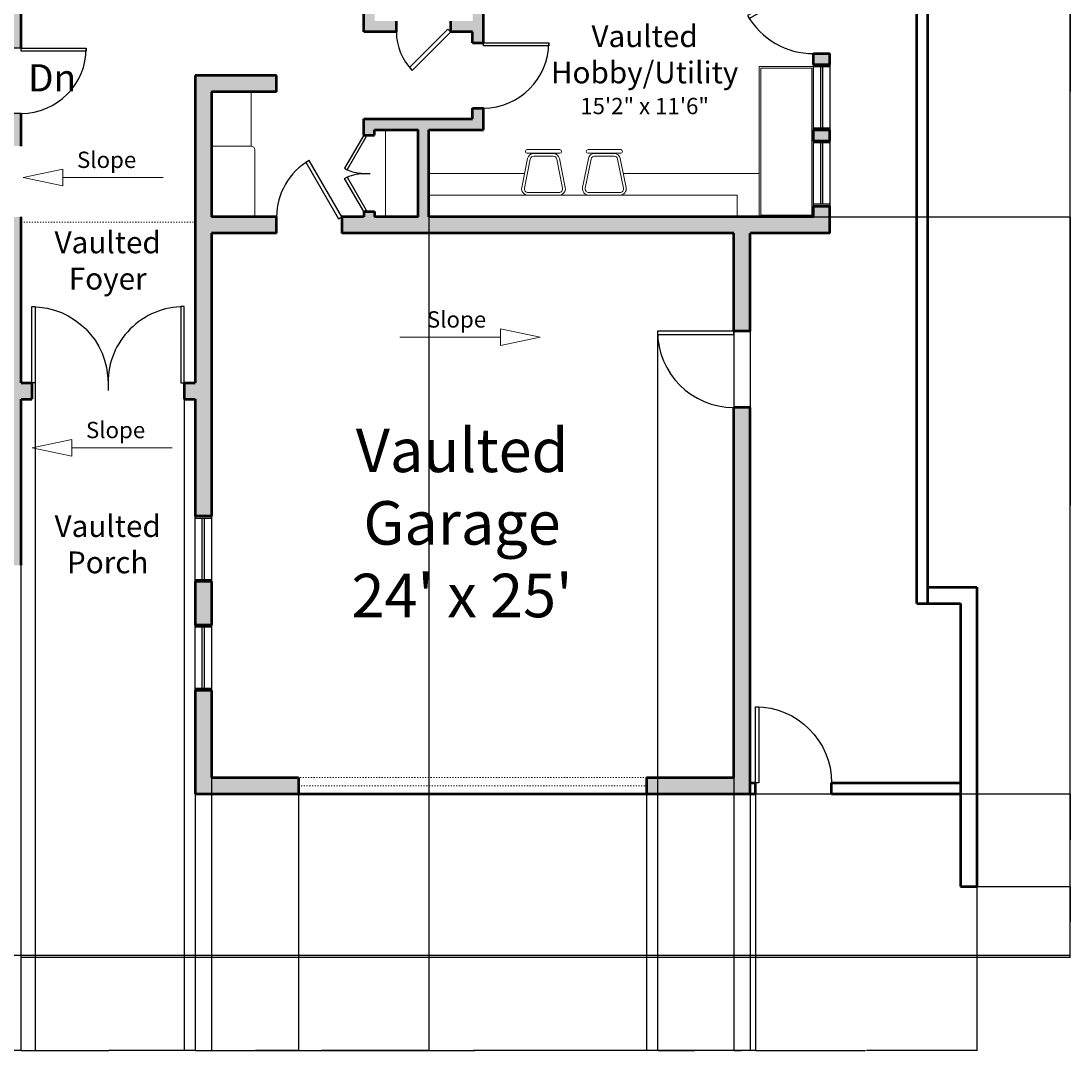
# Model space of a CAD drawing. Units: inches. Extents: x 296 to 2116, y 330 to 1460.
# Tile 2 of 9: x 657 to 1235, y 330 to 898. Entities that reach past the tile are written whole.
import ezdxf

# ---------------------------------------------------------------- set-up
doc = ezdxf.new("R2010")
doc.units = ezdxf.units.IN
doc.linetypes.add('ACAD_ISO03W100', pattern=[30, 12, -18])
for name, color, linetype, lineweight in [('A-ANNO-DIMS', 2, 'Continuous', 18), ('A-ANNO-SYMB', 2, 'Continuous', 18), ('A-ANNO-TEXT', 7, 'Continuous', 18), ('A-AREA-IDEN', 7, 'Continuous', 25), ('A-DOOR', 3, 'Continuous', 25), ('A-FLOR-FIXT', 8, 'Continuous', 18), ('A-FLOR-OVHD', 132, 'ACAD_ISO03W100', 18), ('A-GLAZ', 4, 'Continuous', 25), ('A-WALL', 7, 'Continuous', 50), ('A-WALL-PATT', 8, 'Continuous', 13)]:
    doc.layers.add(name, color=color, linetype=linetype, lineweight=lineweight)
doc.styles.get("Standard").update_dxf_attribs({"font": 'arial.ttf'})
doc.dimstyles.get("Standard").update_dxf_attribs({"dimtxt": 0.18, "dimasz": 0.18, "dimexe": 0.18, "dimexo": 0.0625, "dimgap": 0.09, "dimtad": 0, "dimtih": 1, "dimtoh": 1, "dimdec": 4, "dimzin": 0, "dimdsep": 46, "dimtxsty": 'Standard', "dimcen": 0.09, "dimadec": 0, "dimazin": 0, "dimtfac": 1, "dimtdec": 4, "dimtofl": 0, "dimtmove": 0, "dimatfit": 3, "dimfxl": 1, "dimtolj": 1, "dimtzin": 0, "dimarcsym": 0})

# ---------------------------------------------------------------- blocks, each defined once
blk = doc.blocks.new('*U5')
for p, q in [((0, 0), (0, 4)), ((40, 0), (40, 4))]:
    blk.add_line(p, q)
blk.add_lwpolyline([(0, 0), (0, -40), (1.75, -40), (1.75, 0)], close=True)
blk.add_arc((0, 0), 40, 270, 0)
blk = doc.blocks.new('*U6')
for p, q in [((0, 0), (0, 4)), ((30, 0), (30, 4))]:
    blk.add_line(p, q)
blk.add_lwpolyline([(0, 0), (15, -25.98), (16.52, -25.11), (1.52, 0.88)], close=True)
blk.add_arc((0, 0), 30, 300, 0)
blk = doc.blocks.new('*U8')
for p, q in [((-24, 0), (-24, -4)), ((0, 0), (0, -4))]:
    blk.add_line(p, q)
blk.add_lwpolyline([(0, 0), (-20.78, 12), (-21.66, 10.48), (-0.88, -1.52)], close=True)
blk.add_arc((0, 0), 24, 150, 180)
blk = doc.blocks.new('*U7')
for p, q in [((-36, 0), (-36, 4)), ((0, 0), (0, 4))]:
    blk.add_line(p, q)
blk.add_lwpolyline([(0, 0), (0, -36), (-1.75, -36), (-1.75, 0)], close=True)
blk.add_arc((0, 0), 36, 180, 270)
blk = doc.blocks.new('*U10')
for p, q in [((0, 0), (0, -4)), ((24, 0), (24, -4))]:
    blk.add_line(p, q)
blk.add_lwpolyline([(0, 0), (16.97, 16.97), (18.21, 15.73), (1.24, -1.24)], close=True)
blk.add_arc((0, 0), 24, 0, 45)
blk = doc.blocks.new('*U11')
for p, q in [((0, 0), (0, -4)), ((-40, 0), (-40, -4))]:
    blk.add_line(p, q)
blk.add_lwpolyline([(0, 0), (-20, 34.64), (-21.52, 33.77), (-1.52, -0.88)], close=True)
blk.add_arc((0, 0), 40, 120, 180)
blk = doc.blocks.new('*U12')
for p, q in [((0, 0), (0, -4)), ((-40, 0), (-40, -4))]:
    blk.add_line(p, q)
blk.add_lwpolyline([(0, 0), (0, 40), (-1.75, 40), (-1.75, 0)], close=True)
blk.add_arc((0, 0), 40, 90, 180)
blk = doc.blocks.new('*U15')
for p, q in [((-36, 0), (-36, 6)), ((0, 0), (0, 6))]:
    blk.add_line(p, q)
blk.add_lwpolyline([(0, 0), (0, -36), (-1.75, -36), (-1.75, 0)], close=True)
blk.add_arc((0, 0), 36, 180, 270)
blk = doc.blocks.new('SLOPE-ARROW')
blk.add_line((739.99, 662.71), (684.54, 662.71))
blk.add_lwpolyline([(662.67, 662.71), (684.54, 658.1), (684.54, 667.32)], close=True)
blk = doc.blocks.new('*D45')
at = {"layer": 'A-ANNO-DIMS', "color": 0, "lineweight": -2, "transparency": 16777216}
for p, q in [((1156.58, 1407.95), (1235.3, 1407.95)), ((1235.12, 1407.77), (1235.12, 895.66)), ((1235.12, 383.18), (1235.12, 895.29)), ((609.63, 383), (1235.3, 383))]:
    blk.add_line(p, q, dxfattribs=at)
at = {"layer": 'A-ANNO-DIMS', "color": 0, "transparency": 16777216}
for points in [[(1235.09, 1407.77), (1235.15, 1407.77), (1235.12, 1407.95)], [(1235.09, 383.18), (1235.15, 383.18), (1235.12, 383)]]:
    blk.add_solid(points, dxfattribs=at)
at = {"layer": 'Defpoints', "color": 0, "transparency": 16777216}
for p in [(1156.52, 1407.95), (1235.12, 1407.95), (609.57, 383)]:
    blk.add_point(p, dxfattribs=at)
at = {"layer": 'A-ANNO-DIMS', "color": 0, "transparency": 16777216, "insert": (1235.12, 895.48), "char_height": 0.18, "attachment_point": 5}
blk.add_mtext('\\A1;1025', dxfattribs=at)
blk = doc.blocks.new('*D53')
at = {"layer": 'A-ANNO-DIMS', "color": 0, "lineweight": -2, "transparency": 16777216}
for p, q in [((609.57, 382.94), (609.57, 330.22)), ((656.57, 381.94), (656.57, 330.22)), ((609.75, 330.4), (632.85, 330.4)), ((656.39, 330.4), (633.29, 330.4))]:
    blk.add_line(p, q, dxfattribs=at)
at = {"layer": 'A-ANNO-DIMS', "color": 0, "transparency": 16777216}
for points in [[(609.75, 330.43), (609.75, 330.37), (609.57, 330.4)], [(656.39, 330.43), (656.39, 330.37), (656.57, 330.4)]]:
    blk.add_solid(points, dxfattribs=at)
at = {"layer": 'Defpoints', "color": 0, "transparency": 16777216}
for p in [(609.57, 383), (656.57, 382), (656.57, 330.4)]:
    blk.add_point(p, dxfattribs=at)
at = {"layer": 'A-ANNO-DIMS', "color": 0, "transparency": 16777216, "insert": (633.07, 330.4), "char_height": 0.18, "attachment_point": 5}
blk.add_mtext('\\A1;47', dxfattribs=at)
blk = doc.blocks.new('*D54')
at = {"layer": 'A-ANNO-DIMS', "color": 0, "lineweight": -2, "transparency": 16777216}
for p, q in [((656.57, 597.94), (656.57, 330.22)), ((752.52, 471.89), (752.52, 330.22)), ((656.75, 330.4), (704.15, 330.4)), ((752.34, 330.4), (704.94, 330.4))]:
    blk.add_line(p, q, dxfattribs=at)
at = {"layer": 'A-ANNO-DIMS', "color": 0, "transparency": 16777216}
for points in [[(656.75, 330.43), (656.75, 330.37), (656.57, 330.4)], [(752.34, 330.43), (752.34, 330.37), (752.52, 330.4)]]:
    blk.add_solid(points, dxfattribs=at)
at = {"layer": 'Defpoints', "color": 0, "transparency": 16777216}
for p in [(656.57, 598), (752.52, 471.95), (752.52, 330.4)]:
    blk.add_point(p, dxfattribs=at)
at = {"layer": 'A-ANNO-DIMS', "color": 0, "transparency": 16777216, "insert": (704.55, 330.4), "char_height": 0.18, "attachment_point": 5}
blk.add_mtext('\\A1;95.95', dxfattribs=at)
blk = doc.blocks.new('*D55')
at = {"layer": 'A-ANNO-DIMS', "color": 0, "lineweight": -2, "transparency": 16777216}
for p, q in [((752.52, 471.89), (752.52, 330.22)), ((1061.52, 471.89), (1061.52, 330.22)), ((752.7, 330.4), (906.73, 330.4)), ((1061.34, 330.4), (907.31, 330.4))]:
    blk.add_line(p, q, dxfattribs=at)
at = {"layer": 'A-ANNO-DIMS', "color": 0, "transparency": 16777216}
for points in [[(752.7, 330.43), (752.7, 330.37), (752.52, 330.4)], [(1061.34, 330.43), (1061.34, 330.37), (1061.52, 330.4)]]:
    blk.add_solid(points, dxfattribs=at)
at = {"layer": 'Defpoints', "color": 0, "transparency": 16777216}
for p in [(752.52, 471.95), (1061.52, 471.95), (1061.52, 330.4)]:
    blk.add_point(p, dxfattribs=at)
at = {"layer": 'A-ANNO-DIMS', "color": 0, "transparency": 16777216, "insert": (907.02, 330.4), "char_height": 0.18, "attachment_point": 5}
blk.add_mtext('\\A1;309', dxfattribs=at)
blk = doc.blocks.new('*D56')
at = {"layer": 'A-ANNO-DIMS', "color": 0, "lineweight": -2, "transparency": 16777216}
for p, q in [((1183.52, 585.89), (1183.52, 330.22)), ((1061.52, 471.89), (1061.52, 330.22)), ((1061.7, 330.4), (1122.24, 330.4)), ((1183.34, 330.4), (1122.8, 330.4))]:
    blk.add_line(p, q, dxfattribs=at)
at = {"layer": 'A-ANNO-DIMS', "color": 0, "transparency": 16777216}
for points in [[(1061.7, 330.43), (1061.7, 330.37), (1061.52, 330.4)], [(1183.34, 330.43), (1183.34, 330.37), (1183.52, 330.4)]]:
    blk.add_solid(points, dxfattribs=at)
at = {"layer": 'Defpoints', "color": 0, "transparency": 16777216}
for p in [(1183.52, 585.95), (1061.52, 471.95), (1183.52, 330.4)]:
    blk.add_point(p, dxfattribs=at)
at = {"layer": 'A-ANNO-DIMS', "color": 0, "transparency": 16777216, "insert": (1122.52, 330.4), "char_height": 0.18, "attachment_point": 5}
blk.add_mtext('\\A1;122', dxfattribs=at)
blk = doc.blocks.new('*D60')
at = {"layer": 'A-ANNO-DIMS', "color": 0, "lineweight": -2, "transparency": 16777216}
for p, q in [((1174.58, 420.95), (1235.3, 420.95)), ((1235.12, 420.77), (1235.12, 401.66)), ((1235.12, 382.18), (1235.12, 401.29)), ((656.63, 382), (1235.3, 382))]:
    blk.add_line(p, q, dxfattribs=at)
at = {"layer": 'A-ANNO-DIMS', "color": 0, "transparency": 16777216}
for points in [[(1235.09, 420.77), (1235.15, 420.77), (1235.12, 420.95)], [(1235.09, 382.18), (1235.15, 382.18), (1235.12, 382)]]:
    blk.add_solid(points, dxfattribs=at)
at = {"layer": 'Defpoints', "color": 0, "transparency": 16777216}
for p in [(1174.52, 420.95), (1235.12, 420.95), (656.57, 382)]:
    blk.add_point(p, dxfattribs=at)
at = {"layer": 'A-ANNO-DIMS', "color": 0, "transparency": 16777216, "insert": (1235.12, 401.48), "char_height": 0.18, "attachment_point": 5}
blk.add_mtext('\\A1;38.955', dxfattribs=at)
blk = doc.blocks.new('*D61')
at = {"layer": 'A-ANNO-DIMS', "color": 0, "lineweight": -2, "transparency": 16777216}
for p, q in [((1061.58, 471.95), (1235.3, 471.95)), ((1235.12, 471.77), (1235.12, 446.64)), ((1235.12, 421.13), (1235.12, 446.27)), ((1174.58, 420.95), (1235.3, 420.95))]:
    blk.add_line(p, q, dxfattribs=at)
at = {"layer": 'A-ANNO-DIMS', "color": 0, "transparency": 16777216}
for points in [[(1235.09, 471.77), (1235.15, 471.77), (1235.12, 471.95)], [(1235.09, 421.13), (1235.15, 421.13), (1235.12, 420.95)]]:
    blk.add_solid(points, dxfattribs=at)
at = {"layer": 'Defpoints', "color": 0, "transparency": 16777216}
for p in [(1061.52, 471.95), (1235.12, 471.95), (1174.52, 420.95)]:
    blk.add_point(p, dxfattribs=at)
at = {"layer": 'A-ANNO-DIMS', "color": 0, "transparency": 16777216, "insert": (1235.12, 446.45), "char_height": 0.18, "attachment_point": 5}
blk.add_mtext('\\A1;51', dxfattribs=at)
blk = doc.blocks.new('*D62')
at = {"layer": 'A-ANNO-DIMS', "color": 0, "lineweight": -2, "transparency": 16777216}
for p, q in [((1063.58, 789.95), (1235.3, 789.95)), ((1235.12, 789.77), (1235.12, 631.14)), ((1235.12, 472.13), (1235.12, 630.77)), ((1061.58, 471.95), (1235.3, 471.95))]:
    blk.add_line(p, q, dxfattribs=at)
at = {"layer": 'A-ANNO-DIMS', "color": 0, "transparency": 16777216}
for points in [[(1235.09, 789.77), (1235.15, 789.77), (1235.12, 789.95)], [(1235.09, 472.13), (1235.15, 472.13), (1235.12, 471.95)]]:
    blk.add_solid(points, dxfattribs=at)
at = {"layer": 'Defpoints', "color": 0, "transparency": 16777216}
for p in [(1063.52, 789.95), (1235.12, 789.95), (1061.52, 471.95)]:
    blk.add_point(p, dxfattribs=at)
at = {"layer": 'A-ANNO-DIMS', "color": 0, "transparency": 16777216, "insert": (1235.12, 630.95), "char_height": 0.18, "attachment_point": 5}
blk.add_mtext('\\A1;318', dxfattribs=at)
blk = doc.blocks.new('*D63')
at = {"layer": 'A-ANNO-DIMS', "color": 0, "lineweight": -2, "transparency": 16777216}
for p, q in [((1102.58, 1156.95), (1235.3, 1156.95)), ((1235.12, 1156.77), (1235.12, 973.64)), ((1235.12, 790.13), (1235.12, 973.27)), ((1063.58, 789.95), (1235.3, 789.95))]:
    blk.add_line(p, q, dxfattribs=at)
at = {"layer": 'A-ANNO-DIMS', "color": 0, "transparency": 16777216}
for points in [[(1235.09, 1156.77), (1235.15, 1156.77), (1235.12, 1156.95)], [(1235.09, 790.13), (1235.15, 790.13), (1235.12, 789.95)]]:
    blk.add_solid(points, dxfattribs=at)
at = {"layer": 'Defpoints', "color": 0, "transparency": 16777216}
for p in [(1102.52, 1156.95), (1235.12, 1156.95), (1063.52, 789.95)]:
    blk.add_point(p, dxfattribs=at)
at = {"layer": 'A-ANNO-DIMS', "color": 0, "transparency": 16777216, "insert": (1235.12, 973.45), "char_height": 0.18, "attachment_point": 5}
blk.add_mtext('\\A1;367', dxfattribs=at)
blk = doc.blocks.new('*D76')
at = {"layer": 'A-ANNO-DIMS', "color": 0, "lineweight": -2, "transparency": 16777216}
for p, q in [((1049.52, 780.89), (1049.52, 330.22)), ((1058.52, 780.89), (1058.52, 330.22)), ((1049.7, 330.4), (1053.7, 330.4)), ((1058.34, 330.4), (1054.35, 330.4))]:
    blk.add_line(p, q, dxfattribs=at)
at = {"layer": 'A-ANNO-DIMS', "color": 0, "transparency": 16777216}
for points in [[(1049.7, 330.43), (1049.7, 330.37), (1049.52, 330.4)], [(1058.34, 330.43), (1058.34, 330.37), (1058.52, 330.4)]]:
    blk.add_solid(points, dxfattribs=at)
at = {"layer": 'Defpoints', "color": 0, "transparency": 16777216}
for p in [(1049.52, 780.95), (1058.52, 780.95), (1058.52, 330.4)]:
    blk.add_point(p, dxfattribs=at)
at = {"layer": 'A-ANNO-DIMS', "color": 0, "transparency": 16777216, "insert": (1054.02, 330.4), "char_height": 0.18, "attachment_point": 5}
blk.add_mtext('\\A1;9.00', dxfattribs=at)
blk = doc.blocks.new('*D95')
at = {"layer": 'A-ANNO-DIMS', "color": 0, "lineweight": -2, "transparency": 16777216}
for p, q in [((761.52, 480.89), (761.52, 330.22)), ((809.52, 480.89), (809.52, 330.22)), ((761.7, 330.4), (785.13, 330.4)), ((809.34, 330.4), (785.92, 330.4))]:
    blk.add_line(p, q, dxfattribs=at)
at = {"layer": 'A-ANNO-DIMS', "color": 0, "transparency": 16777216}
for points in [[(761.7, 330.43), (761.7, 330.37), (761.52, 330.4)], [(809.34, 330.43), (809.34, 330.37), (809.52, 330.4)]]:
    blk.add_solid(points, dxfattribs=at)
at = {"layer": 'Defpoints', "color": 0, "transparency": 16777216}
for p in [(761.52, 480.95), (809.52, 480.95), (809.52, 330.4)]:
    blk.add_point(p, dxfattribs=at)
at = {"layer": 'A-ANNO-DIMS', "color": 0, "transparency": 16777216, "insert": (785.52, 330.4), "char_height": 0.18, "attachment_point": 5}
blk.add_mtext('\\A1;48.00', dxfattribs=at)
blk = doc.blocks.new('*D96')
at = {"layer": 'A-ANNO-DIMS', "color": 0, "lineweight": -2, "transparency": 16777216}
for p, q in [((809.52, 480.89), (809.52, 330.22)), ((1001.52, 480.89), (1001.52, 330.22)), ((809.7, 330.4), (905.07, 330.4)), ((1001.34, 330.4), (905.98, 330.4))]:
    blk.add_line(p, q, dxfattribs=at)
at = {"layer": 'A-ANNO-DIMS', "color": 0, "transparency": 16777216}
for points in [[(809.7, 330.43), (809.7, 330.37), (809.52, 330.4)], [(1001.34, 330.43), (1001.34, 330.37), (1001.52, 330.4)]]:
    blk.add_solid(points, dxfattribs=at)
at = {"layer": 'Defpoints', "color": 0, "transparency": 16777216}
for p in [(809.52, 480.95), (1001.52, 480.95), (1001.52, 330.4)]:
    blk.add_point(p, dxfattribs=at)
at = {"layer": 'A-ANNO-DIMS', "color": 0, "transparency": 16777216, "insert": (905.52, 330.4), "char_height": 0.18, "attachment_point": 5}
blk.add_mtext('\\A1;192.00', dxfattribs=at)
blk = doc.blocks.new('*D97')
at = {"layer": 'A-ANNO-DIMS', "color": 0, "lineweight": -2, "transparency": 16777216}
for p, q in [((881.52, 789.89), (881.52, 330.22)), ((761.52, 780.89), (761.52, 330.22)), ((761.7, 330.4), (821.07, 330.4)), ((881.34, 330.4), (821.98, 330.4))]:
    blk.add_line(p, q, dxfattribs=at)
at = {"layer": 'A-ANNO-DIMS', "color": 0, "transparency": 16777216}
for points in [[(761.7, 330.43), (761.7, 330.37), (761.52, 330.4)], [(881.34, 330.43), (881.34, 330.37), (881.52, 330.4)]]:
    blk.add_solid(points, dxfattribs=at)
at = {"layer": 'Defpoints', "color": 0, "transparency": 16777216}
for p in [(881.52, 789.95), (761.52, 780.95), (881.52, 330.4)]:
    blk.add_point(p, dxfattribs=at)
at = {"layer": 'A-ANNO-DIMS', "color": 0, "transparency": 16777216, "insert": (821.52, 330.4), "char_height": 0.18, "attachment_point": 5}
blk.add_mtext('\\A1;120.00', dxfattribs=at)
blk = doc.blocks.new('*D98')
at = {"layer": 'A-ANNO-DIMS', "color": 0, "lineweight": -2, "transparency": 16777216}
for p, q in [((1030.58, 927.95), (1235.3, 927.95)), ((1235.12, 927.77), (1235.12, 859.14)), ((1235.12, 790.13), (1235.12, 858.77)), ((1093.58, 789.95), (1235.3, 789.95))]:
    blk.add_line(p, q, dxfattribs=at)
at = {"layer": 'A-ANNO-DIMS', "color": 0, "transparency": 16777216}
for points in [[(1235.09, 927.77), (1235.15, 927.77), (1235.12, 927.95)], [(1235.09, 790.13), (1235.15, 790.13), (1235.12, 789.95)]]:
    blk.add_solid(points, dxfattribs=at)
at = {"layer": 'Defpoints', "color": 0, "transparency": 16777216}
for p in [(1030.52, 927.95), (1235.12, 927.95), (1093.52, 789.95)]:
    blk.add_point(p, dxfattribs=at)
at = {"layer": 'A-ANNO-DIMS', "color": 0, "transparency": 16777216, "insert": (1235.12, 858.95), "char_height": 0.18, "attachment_point": 5}
blk.add_mtext('\\A1;138.00', dxfattribs=at)
blk = doc.blocks.new('*D99')
at = {"layer": 'A-ANNO-DIMS', "color": 0, "lineweight": -2, "transparency": 16777216}
for p, q in [((664.38, 698.44), (664.38, 330.22)), ((746.55, 698.44), (746.55, 330.22)), ((664.56, 330.4), (705.07, 330.4)), ((746.37, 330.4), (705.86, 330.4))]:
    blk.add_line(p, q, dxfattribs=at)
at = {"layer": 'A-ANNO-DIMS', "color": 0, "transparency": 16777216}
for points in [[(664.56, 330.43), (664.56, 330.37), (664.38, 330.4)], [(746.37, 330.43), (746.37, 330.37), (746.55, 330.4)]]:
    blk.add_solid(points, dxfattribs=at)
at = {"layer": 'Defpoints', "color": 0, "transparency": 16777216}
for p in [(664.38, 698.5), (746.55, 698.5), (746.55, 330.4)]:
    blk.add_point(p, dxfattribs=at)
at = {"layer": 'A-ANNO-DIMS', "color": 0, "transparency": 16777216, "insert": (705.47, 330.4), "char_height": 0.18, "attachment_point": 5}
blk.add_mtext('\\A1;82.16', dxfattribs=at)
blk = doc.blocks.new('*D101')
at = {"layer": 'A-ANNO-DIMS', "color": 0, "lineweight": -2, "transparency": 16777216}
for p, q in [((1007.52, 726.89), (1007.52, 330.22)), ((1049.52, 726.89), (1049.52, 330.22)), ((1007.7, 330.4), (1028.13, 330.4)), ((1049.34, 330.4), (1028.92, 330.4))]:
    blk.add_line(p, q, dxfattribs=at)
at = {"layer": 'A-ANNO-DIMS', "color": 0, "transparency": 16777216}
for points in [[(1007.7, 330.43), (1007.7, 330.37), (1007.52, 330.4)], [(1049.34, 330.43), (1049.34, 330.37), (1049.52, 330.4)]]:
    blk.add_solid(points, dxfattribs=at)
at = {"layer": 'Defpoints', "color": 0, "transparency": 16777216}
for p in [(1007.52, 726.95), (1049.52, 726.95), (1049.52, 330.4)]:
    blk.add_point(p, dxfattribs=at)
at = {"layer": 'A-ANNO-DIMS', "color": 0, "transparency": 16777216, "insert": (1028.52, 330.4), "char_height": 0.18, "attachment_point": 5}
blk.add_mtext('\\A1;42.00', dxfattribs=at)

msp = doc.modelspace()

# ---------------------------------------------------------------- hatches: boundary and pattern name
at = {"layer": 'A-WALL-PATT'}
h = msp.add_hatch(color=256, dxfattribs=at)
h.dxf.hatch_style = 1
h.paths.add_polyline_path([(656.5723, 927.9991), (668.5723, 927.9991), (668.5723, 936.9991), (650.5723, 936.9991), (650.5723, 897.9991), (356.5223, 897.9991), (356.5223, 955.9991), (347.5223, 955.9991), (347.5223, 888.9991), (423.5723, 888.9991), (423.5723, 766.9991), (432.5723, 766.9991), (432.5723, 834.9991), (453.5723, 834.9991), (468.5723, 834.9991), (468.5723, 840.9991), (432.5723, 840.9991), (432.5723, 888.9991), (504.5723, 888.9991), (504.5723, 840.9991), (504.5723, 834.9991), (531.6223, 834.9991), (531.6223, 768.5344), (527.8443, 764.7564), (530.6728, 761.928), (532.087, 760.5138), (540.5723, 768.9991), (598.0723, 768.9991), (598.0723, 777.9991), (601.8223, 777.9991), (601.8223, 782.1991), (601.8223, 783.9991), (598.0723, 783.9991), (598.0723, 798.9991), (592.0723, 798.9991), (592.0723, 774.9991), (537.6223, 774.9991), (537.6223, 834.9991), (592.0723, 834.9991), (592.0723, 828.9991), (598.0723, 828.9991), (598.0723, 834.9991), (647.5723, 834.9991), (647.5723, 828.9991), (656.5723, 828.9991), (656.5723, 846.9991), (650.5723, 846.9991), (647.5723, 846.9991), (647.5723, 840.9991), (510.5723, 840.9991), (510.5723, 888.9991), (647.5723, 888.9991), (647.5723, 882.9991), (656.5723, 882.9991)])
h.paths.add_polyline_path([(432.5723, 730.9991), (496.5723, 730.9991), (496.5723, 724.9991), (502.5723, 724.9991), (502.5723, 730.9991), (506.6311, 735.058), (502.3885, 739.3006), (500.087, 736.9991), (432.5723, 736.9991), (432.5723, 742.9991), (423.5723, 742.9991), (423.5723, 641.9991), (490.5723, 641.9991), (490.5723, 597.9991), (531.5723, 597.9991), (531.5723, 606.9991), (499.5723, 606.9991), (499.5723, 650.9991), (502.5723, 650.9991), (502.5723, 659.9991), (496.5723, 659.9991), (493.5723, 659.9991), (493.5723, 650.9991), (432.5723, 650.9991)])
h.paths.add_polyline_path([(656.5723, 689.4991), (662.5473, 689.4991), (662.5473, 698.4991), (656.5723, 698.4991), (656.5723, 789.9991), (647.5723, 789.9991), (647.5723, 783.9991), (643.8223, 783.9991), (643.8223, 777.9991), (647.5723, 777.9991), (647.5723, 606.9991), (615.5723, 606.9991), (615.5723, 597.9991), (656.5723, 597.9991)])
h.paths.add_polyline_path([(761.5223, 780.9541), (797.5223, 780.9541), (797.5223, 789.9541), (761.5223, 789.9541), (761.5223, 858.9541), (797.5223, 858.9541), (797.5223, 867.9541), (752.5223, 867.9541), (752.5223, 698.4991), (746.5473, 698.4991), (746.5473, 694.2991), (746.5473, 689.4991), (752.5223, 689.4991), (752.5223, 624.9541), (761.5223, 624.9541)])
h.paths.add_polyline_path([(1102.5223, 795.9541), (1093.5223, 795.9541), (1093.5223, 789.9541), (1063.5223, 789.9541), (881.5223, 789.9541), (881.5223, 837.9541), (911.5223, 837.9541), (911.5223, 849.9541), (907.5223, 849.9541), (905.5223, 849.9541), (905.5223, 843.9541), (845.5223, 843.9541), (845.5223, 834.9541), (849.0223, 834.9541), (851.5223, 834.9541), (851.5223, 837.9541), (875.5223, 837.9541), (875.5223, 789.9541), (851.5223, 789.9541), (851.5223, 792.9541), (845.5223, 792.9541), (845.5223, 789.9541), (833.5223, 789.9541), (833.5223, 785.1541), (833.5223, 780.9541), (1049.5223, 780.9541), (1049.5223, 726.9541), (1053.7223, 726.9541), (1058.5223, 726.9541), (1058.5223, 780.9541), (1102.5223, 780.9541)])
h.paths.add_polyline_path([(761.5223, 588.9541), (752.5223, 588.9541), (752.5223, 564.9541), (761.5223, 564.9541)])
h.paths.add_polyline_path([(809.5223, 480.9541), (761.5223, 480.9541), (761.5223, 528.9541), (752.5223, 528.9541), (752.5223, 471.9541), (809.5223, 471.9541)])
h.paths.add_polyline_path([(1058.5223, 684.9541), (1049.5223, 684.9541), (1049.5223, 480.9541), (1001.5223, 480.9541), (1001.5223, 476.4541), (1001.5223, 471.9541), (1058.5223, 471.9541)])
h.paths.add_polyline_path([(794.5223, 1013.9991), (800.5223, 1013.9991), (800.5223, 1019.9991), (794.5223, 1019.9991), (794.5223, 1296.9541), (785.5223, 1296.9541), (785.5223, 1221.9991), (752.5223, 1221.9991), (752.5223, 1212.9991), (788.5223, 1212.9991), (788.5223, 936.9991), (752.5223, 936.9991), (752.5223, 927.9991), (794.5223, 927.9991)])
h.paths.add_polyline_path([(450.0223, 1191.9991), (398.5223, 1191.9991), (398.5223, 1137.9991), (407.5223, 1137.9991), (407.5223, 1182.9991), (450.0223, 1182.9991)])
h.paths.add_polyline_path([(576.5223, 1212.9991), (612.5223, 1212.9991), (612.5223, 1221.9991), (567.5223, 1221.9991), (567.5223, 1191.9991), (540.0223, 1191.9991), (540.0223, 1182.9991), (576.5223, 1182.9991)])
h.paths.add_polyline_path([(407.5223, 1060.9991), (398.5223, 1060.9991), (398.5223, 1030.9991), (392.5223, 1030.9991), (392.5223, 1021.9991), (407.5223, 1021.9991)])
h.paths.add_polyline_path([(356.5223, 1030.9991), (347.5223, 1030.9991), (347.5223, 1015.9991), (356.5223, 1015.9991), (356.5223, 1021.9991)])
h.paths.add_polyline_path([(788.5223, 1129.9991), (770.0334, 1131.3572, 0.43585667), (767.8869, 1129.3626), (767.8869, 1108.3618, 0.31855172), (769.8942, 1105.5308), (788.5223, 1098.9991)], flags=17)
h.paths.add_polyline_path([(788.5223, 1050.9991), (769.8942, 1044.4674, 0.31855172), (767.8869, 1041.6364), (767.8869, 1020.6356, 0.43585667), (770.0334, 1018.641), (788.5223, 1019.9991)], flags=17)
h.paths.add_polyline_path([(893.5223, 1066.9541), (851.5223, 1066.9541), (851.5223, 1069.9541), (845.5223, 1069.9541), (845.5223, 1019.9991), (839.5223, 1019.9991), (839.5223, 1013.9991), (845.5223, 1013.9991), (845.5223, 891.9541), (863.5223, 891.9541), (863.5223, 897.9541), (851.5223, 897.9541), (851.5223, 927.9541), (905.5223, 927.9541), (905.5223, 897.9541), (893.5223, 897.9541), (893.5223, 891.9541), (905.5223, 891.9541), (905.5223, 885.9541), (911.5223, 885.9541), (911.5223, 927.9541), (1030.5223, 927.9541), (1030.5223, 936.9541), (1013.5223, 936.9541), (1013.5223, 996.9541), (1093.5223, 996.9541), (1093.5223, 936.9541), (1066.5223, 936.9541), (1066.5223, 927.9541), (1093.5223, 927.9541), (1093.5223, 921.9541), (1102.5223, 921.9541), (1102.5223, 1013.9541), (1093.5223, 1013.9541), (1093.5223, 1002.9541), (1013.5223, 1002.9541), (1013.5223, 1060.9541), (1013.5223, 1066.9541), (1007.5223, 1066.9541), (1007.5223, 1042.9541), (977.5223, 1042.9541), (977.5223, 1066.9541), (965.5223, 1066.9541), (965.5223, 1060.9541), (971.5223, 1060.9541), (971.5223, 1036.9541), (1007.5223, 1036.9541), (1007.5223, 936.9541), (851.5223, 936.9541), (851.5223, 1060.9541), (893.5223, 1060.9541)])
h.paths.add_polyline_path([(851.5223, 1150.9541), (919.5223, 1150.9541), (919.5223, 1114.9541), (911.5223, 1114.9541), (911.5223, 1108.9541), (925.5223, 1108.9541), (925.5223, 1150.9541), (1007.5223, 1150.9541), (1007.5223, 1114.9541), (1013.5223, 1114.9541), (1013.5223, 1150.9541), (1046.5223, 1150.9541), (1046.5223, 1159.9541), (1007.5223, 1159.9541), (1007.5223, 1186.9541), (998.5223, 1186.9541), (998.5223, 1156.9541), (845.5223, 1156.9541), (845.5223, 1105.9541), (851.5223, 1105.9541)])
h.paths.add_polyline_path([(1102.5223, 1156.9541), (1102.5223, 1159.9541), (1088.5223, 1159.9541), (1088.5223, 1150.9541), (1093.5223, 1150.9541), (1093.5223, 1147.9541), (1102.5223, 1147.9541)])
h.paths.add_polyline_path([(1102.5223, 1111.9541), (1093.5223, 1111.9541), (1093.5223, 1066.9541), (1047.5223, 1066.9541), (1047.5223, 1030.9541), (1053.5223, 1030.9541), (1053.5223, 1060.9541), (1093.5223, 1060.9541), (1093.5223, 1049.9541), (1102.5223, 1049.9541)])
h.paths.add_polyline_path([(1102.5223, 837.9541), (1093.5223, 837.9541), (1093.5223, 831.9541), (1102.5223, 831.9541)], flags=17)
h.paths.add_polyline_path([(1102.5223, 879.9541), (1093.5223, 879.9541), (1093.5223, 873.9541), (1102.5223, 873.9541)])
h.paths.add_polyline_path([(839.5223, 1353.9541), (785.5223, 1353.9541), (785.5223, 1338.9541), (794.5223, 1338.9541), (794.5223, 1344.9541), (839.5223, 1344.9541)])
h.paths.add_polyline_path([(1007.5223, 1353.9541), (953.5223, 1353.9541), (953.5223, 1344.9541), (998.5223, 1344.9541), (998.5223, 1314.9541), (1007.5223, 1314.9541)])
h.paths.add_polyline_path([(917.5223, 1353.9541), (914.5223, 1353.9541), (914.5223, 1344.9541), (917.5223, 1344.9541)])
h.paths.add_polyline_path([(878.5223, 1353.9541), (875.5223, 1353.9541), (875.5223, 1344.9541), (878.5223, 1344.9541)])
h.paths.add_polyline_path([(1007.5223, 1278.9541), (998.5223, 1278.9541), (998.5223, 1222.9541), (1007.5223, 1222.9541)])
h.paths.add_polyline_path([(407.5223, 1101.9991), (398.5223, 1101.9991), (398.5223, 1096.9991), (407.5223, 1096.9991)])
h.paths.add_polyline_path([(560.5723, 606.9991), (557.5723, 606.9991), (557.5723, 597.9991), (560.5723, 597.9991)])
h.paths.add_polyline_path([(589.5723, 606.9991), (586.5723, 606.9991), (586.5723, 597.9991), (589.5723, 597.9991)])

# ---------------------------------------------------------------- linework, layer by layer
at = {"layer": 'A-FLOR-FIXT'}
for p, q in [((783.5223, 858.9541), (783.5223, 828.9541)), ((857.5223, 789.9541), (857.5223, 837.9541)), ((783.5223, 828.9541), (761.5223, 828.9541)), ((785.5223, 826.9541), (785.5223, 789.9541)), ((881.5223, 813.9541), (934.2215, 813.9541)), ((988.6477, 813.9541), (1063.5223, 813.9541)), ((881.5223, 801.9541), (1051.5223, 801.9541)), ((1051.5223, 801.9541), (1051.5223, 789.9541))]:
    msp.add_line(p, q, dxfattribs=at)
for points in [[(1063.5223, 789.9541), (1093.5223, 789.9541), (1093.5223, 872.9541), (1063.5223, 872.9541)], [(1064.5223, 790.9541), (1092.5223, 790.9541), (1092.5223, 871.9541), (1064.5223, 871.9541)]]:
    msp.add_lwpolyline(points, close=True, dxfattribs=at)
for points in [[(932.6587, 806.1405, 0.47328482), (936.0908, 801.9541), (953.2116, 801.9541, 0.47328482), (956.6436, 806.1405), (953.4436, 822.1405, 0.35751077), (950.0116, 824.9541), (939.2908, 824.9541, 0.35751077), (935.8587, 822.1405)], [(934.1296, 805.8463, 0.47328482), (936.0908, 803.4541), (953.2116, 803.4541, 0.47328482), (955.1727, 805.8463), (951.9727, 821.8463, 0.35751077), (950.0116, 823.4541), (939.2908, 823.4541, 0.35751077), (937.3296, 821.8463)], [(935.6512, 825.074), (953.6512, 825.074, 1), (953.6512, 827.074), (935.6512, 827.074, 1)], [(966.2255, 806.1405, 0.47328482), (969.6576, 801.9541), (986.7784, 801.9541, 0.47328482), (990.2104, 806.1405), (987.0104, 822.1405, 0.35751077), (983.5784, 824.9541), (972.8576, 824.9541, 0.35751077), (969.4255, 822.1405)], [(967.6964, 805.8463, 0.47328482), (969.6576, 803.4541), (986.7784, 803.4541, 0.47328482), (988.7395, 805.8463), (985.5395, 821.8463, 0.35751077), (983.5784, 823.4541), (972.8576, 823.4541, 0.35751077), (970.8964, 821.8463)], [(969.218, 825.074), (987.218, 825.074, 1), (987.218, 827.074), (969.218, 827.074, 1)]]:
    msp.add_lwpolyline(points, format="xyb", close=True, dxfattribs=at)
msp.add_arc((783.5223, 826.9541), 2, 0, 90, dxfattribs=at)
at = {"layer": 'A-FLOR-OVHD', "ltscale": 0.05}
msp.add_line((656.5723, 787.021), (752.5223, 787.021), dxfattribs=at)
msp.add_lwpolyline([(809.5223, 476.4541), (1001.5223, 476.4541), (1001.5223, 480.9541), (809.5223, 480.9541)], close=True, dxfattribs=at)
at = {"layer": 'A-GLAZ'}
for p, q in [((1093.5223, 872.9541), (1102.5223, 872.9541)), ((1097.5223, 838.9541), (1097.5223, 872.9541)), ((1098.5223, 872.9541), (1098.5223, 838.9541)), ((1102.5223, 838.9541), (1093.5223, 838.9541)), ((1093.5223, 830.9541), (1102.5223, 830.9541)), ((1097.5223, 796.9541), (1097.5223, 830.9541)), ((1098.5223, 830.9541), (1098.5223, 796.9541)), ((1102.5223, 796.9541), (1093.5223, 796.9541)), ((752.5223, 623.9541), (761.5223, 623.9541)), ((756.5223, 589.9541), (756.5223, 623.9541)), ((757.5223, 623.9541), (757.5223, 589.9541)), ((761.5223, 589.9541), (752.5223, 589.9541)), ((752.5223, 563.9541), (761.5223, 563.9541)), ((756.5223, 529.9541), (756.5223, 563.9541)), ((757.5223, 563.9541), (757.5223, 529.9541)), ((761.5223, 529.9541), (752.5223, 529.9541))]:
    msp.add_line(p, q, dxfattribs=at)
for points in [[(1102.5223, 837.9541), (1093.5223, 837.9541), (1093.5223, 873.9541), (1102.5223, 873.9541)], [(1102.5223, 795.9541), (1093.5223, 795.9541), (1093.5223, 831.9541), (1102.5223, 831.9541)], [(761.5223, 588.9541), (752.5223, 588.9541), (752.5223, 624.9541), (761.5223, 624.9541)], [(761.5223, 528.9541), (752.5223, 528.9541), (752.5223, 564.9541), (761.5223, 564.9541)]]:
    msp.add_lwpolyline(points, close=True, dxfattribs=at)
at = {"layer": 'A-WALL'}
for p, q in [((1156.5223, 576.9541), (1156.5223, 1407.9541)), ((1150.5223, 576.9541), (1150.5223, 1066.9541)), ((845.5223, 891.9541), (845.5223, 1013.9991)), ((656.5723, 882.9991), (656.5723, 927.9991)), ((911.5223, 885.9541), (911.5223, 927.9541)), ((863.5223, 891.9541), (863.5223, 897.9541)), ((893.5223, 891.9541), (893.5223, 897.9541)), ((863.5223, 891.9541), (845.5223, 891.9541)), ((905.5223, 891.9541), (893.5223, 891.9541)), ((905.5223, 885.9541), (905.5223, 891.9541)), ((905.5223, 885.9541), (911.5223, 885.9541)), ((1093.5223, 879.9541), (1102.5223, 879.9541)), ((1093.5223, 873.9541), (1093.5223, 879.9541)), ((1102.5223, 873.9541), (1102.5223, 879.9541)), ((1093.5223, 873.9541), (1102.5223, 873.9541)), ((797.5223, 867.9541), (752.5223, 867.9541)), ((752.5223, 867.9541), (752.5223, 698.4991)), ((797.5223, 858.9541), (797.5223, 867.9541)), ((761.5223, 858.9541), (761.5223, 789.9541)), ((797.5223, 858.9541), (761.5223, 858.9541)), ((656.5723, 828.9991), (656.5723, 846.9991)), ((905.5223, 849.9541), (911.5223, 849.9541)), ((905.5223, 843.9541), (905.5223, 849.9541)), ((911.5223, 837.9541), (911.5223, 849.9541)), ((845.5223, 834.9541), (845.5223, 843.9541)), ((845.5223, 843.9541), (905.5223, 843.9541)), ((845.5223, 834.9541), (851.5223, 834.9541)), ((851.5223, 834.9541), (851.5223, 837.9541)), ((851.5223, 837.9541), (875.5223, 837.9541)), ((875.5223, 789.9541), (875.5223, 837.9541)), ((881.5223, 789.9541), (881.5223, 837.9541)), ((881.5223, 837.9541), (911.5223, 837.9541)), ((1093.5223, 837.9541), (1102.5223, 837.9541)), ((1093.5223, 831.9541), (1093.5223, 837.9541)), ((1102.5223, 831.9541), (1102.5223, 837.9541)), ((1093.5223, 831.9541), (1102.5223, 831.9541)), ((1093.5223, 789.9541), (1093.5223, 795.9541)), ((1093.5223, 795.9541), (1102.5223, 795.9541)), ((1102.5223, 780.9541), (1102.5223, 795.9541)), ((656.5723, 698.4991), (656.5723, 789.9991)), ((797.5223, 789.9541), (761.5223, 789.9541)), ((797.5223, 780.9541), (797.5223, 789.9541)), ((833.5223, 789.9541), (833.5223, 780.9541)), ((845.5223, 789.9541), (833.5223, 789.9541)), ((845.5223, 792.9541), (845.5223, 789.9541)), ((845.5223, 792.9541), (851.5223, 792.9541)), ((851.5223, 792.9541), (851.5223, 789.9541)), ((875.5223, 789.9541), (851.5223, 789.9541)), ((1093.5223, 789.9541), (881.5223, 789.9541)), ((797.5223, 780.9541), (761.5223, 780.9541)), ((761.5223, 780.9541), (761.5223, 624.9541)), ((1049.5223, 780.9541), (833.5223, 780.9541)), ((1049.5223, 726.9541), (1049.5223, 780.9541)), ((1102.5223, 780.9541), (1058.5223, 780.9541)), ((1058.5223, 726.9541), (1058.5223, 780.9541)), ((1058.5223, 726.9541), (1049.5223, 726.9541)), ((656.5723, 698.4991), (662.5473, 698.4991)), ((662.5473, 698.4991), (662.5473, 689.4991)), ((746.5473, 698.4991), (746.5473, 689.4991)), ((746.5473, 698.4991), (752.5223, 698.4991)), ((656.5723, 597.9991), (656.5723, 689.4991)), ((656.5723, 689.4991), (662.5473, 689.4991)), ((746.5473, 689.4991), (752.5223, 689.4991)), ((752.5223, 689.4991), (752.5223, 624.9541)), ((1049.5223, 480.9541), (1049.5223, 684.9541)), ((1058.5223, 684.9541), (1049.5223, 684.9541)), ((1058.5223, 471.9541), (1058.5223, 684.9541)), ((761.5223, 624.9541), (752.5223, 624.9541)), ((761.5223, 588.9541), (752.5223, 588.9541)), ((752.5223, 588.9541), (752.5223, 564.9541)), ((761.5223, 588.9541), (761.5223, 564.9541)), ((1156.5223, 585.9541), (1183.5223, 585.9541)), ((1183.5223, 585.9541), (1183.5223, 420.9541)), ((1150.5223, 576.9541), (1174.5223, 576.9541)), ((1174.5223, 576.9541), (1174.5223, 420.9541)), ((761.5223, 564.9541), (752.5223, 564.9541)), ((761.5223, 528.9541), (752.5223, 528.9541)), ((752.5223, 528.9541), (752.5223, 471.9541)), ((761.5223, 528.9541), (761.5223, 480.9541)), ((761.5223, 480.9541), (809.5223, 480.9541)), ((809.5223, 480.9541), (809.5223, 471.9541)), ((1001.5223, 480.9541), (1001.5223, 471.9541)), ((1001.5223, 480.9541), (1049.5223, 480.9541)), ((1058.5223, 477.9541), (1061.5223, 477.9541)), ((1061.5223, 471.9541), (1061.5223, 477.9541)), ((1103.5223, 471.9541), (1103.5223, 477.9541)), ((1103.5223, 477.9541), (1174.5223, 477.9541)), ((752.5223, 471.9541), (1058.5223, 471.9541)), ((1058.5223, 471.9541), (1061.5223, 471.9541)), ((1103.5223, 471.9541), (1174.5223, 471.9541)), ((1174.5223, 420.9541), (1183.5223, 420.9541))]:
    msp.add_line(p, q, dxfattribs=at)

# ---------------------------------------------------------------- block references
at = {"layer": 'A-ANNO-SYMB'}
for p in [(-4.9489, 148.9487), (0, 0)]:
    msp.add_blockref('SLOPE-ARROW', p, dxfattribs=at)
at = {"layer": 'A-ANNO-SYMB', "rotation": 180}
msp.add_blockref('SLOPE-ARROW', (1605.4152, 1386.385), dxfattribs=at)
at = {"layer": 'A-DOOR'}
for name, p, xscale, yscale, zscale, rotation in [('*U11', (1093.5223, 921.9541), 1.05, 1.05, 1.05, 90.00000000000003), ('*U10', (893.5223, 891.9541), 1.250000000000001, 1.250000000000001, 1.250000000000001, 180), ('*U8', (845.5223, 834.9541), 0.8750000000000003, 0.8750000000000003, 0.8750000000000003, 90.00000000000003), ('*U6', (833.5223, 789.9541), 1.199999999999999, 1.199999999999999, 1.199999999999999, 180), ('*U8', (845.5223, 792.9541), -0.8750000000000003, 0.8750000000000003, 0.8750000000000003, 90), ('*U5', (662.5473, 698.4991), -1.05, 1.05, 1.05, 180), ('*U5', (746.5473, 698.4991), 1.05, 1.05, 1.05, 180), ('*U12', (1049.5223, 726.9541), 1.05, 1.05, 1.05, 90.00000000000003), ('*U5', (1061.5223, 477.9541), -1.05, 1.05, 1.05, 180)]:
    msp.add_blockref(name, p, dxfattribs=dict(at, xscale=xscale, yscale=yscale, zscale=zscale, rotation=rotation))
at = {"layer": 'A-DOOR', "rotation": 90.00000000000003}
for name, p in [('*U7', (911.5223, 885.9541)), ('*U15', (656.5723, 882.9991))]:
    msp.add_blockref(name, p, dxfattribs=at)

# ---------------------------------------------------------------- texts
at = {"layer": 'A-ANNO-TEXT'}
for s, width, insert, char_height, attachment_point in [('{\\fArial|b1|i0|c0|p34;Dn}', 22.506546, (660.4594, 874.1411), 15, 1), ('\\pxqc;Slope', 41.969454, (682.785, 825.9476), 9, 1), ('\\pxqc;Slope', 41.969454, (917.6812, 737.9687), 9, 3), ('\\pxqc;Slope', 41.969454, (687.734, 676.9988), 9, 1)]:
    msp.add_mtext_dynamic_manual_height_columns(s, width=width, gutter_width=12.5, heights=[0], dxfattribs=dict(at, insert=insert, char_height=char_height, attachment_point=attachment_point))
at = {"layer": 'A-AREA-IDEN', "attachment_point": 1}
for s, width, insert, char_height in [('\\pxqc;Vaulted\\P{\\fArial|b1|i0|c0|p34;Hobby/Utility\\P\\fArial|b0|i0|c0|p34;\\H0.75x;15\'2" x 11\'6"}', 106.561727, (947.1169, 895.589), 12), ('\\pxqc;Vaulted\\P{\\fArial|b1|i0|c0|p34;Foyer}', 84.176949, (662.2862, 781.9321), 12), ("\\pxqc;Vaulted\\P{\\fArial|b1|i0|c0|p34;Garage\\P}24' x 25'", 167.942646, (815.778, 673.3022), 24), ('\\pxqc;Vaulted\\P{\\fArial|b1|i0|c0|p34;Porch}', 84.176949, (662.2862, 625.5516), 12)]:
    msp.add_mtext_dynamic_manual_height_columns(s, width=width, gutter_width=12.5, heights=[0], dxfattribs=dict(at, insert=insert, char_height=char_height))

# ---------------------------------------------------------------- dimensions: what is measured, and where the dimension line sits
at = {"layer": 'A-ANNO-DIMS'}
for base, p1, p2, override, picture, middle in [((1235.1223, 1407.9541), (609.5723, 382.9991), (1156.5223, 1407.9541), {"dimdec": 0, "dimlfac": 1, "dimrnd": 0, "dimzin": 0, "dimdsep": 46, "dimlunit": 2}, '*D45', (1235.1223, 895.4766)), ((1235.1223, 1156.9541), (1063.5223, 789.9541), (1102.5223, 1156.9541), {"dimdec": 0, "dimlfac": 1, "dimrnd": 0, "dimzin": 0, "dimdsep": 46, "dimlunit": 2}, '*D63', (1235.1223, 973.4541)), ((1235.1223, 927.9541), (1093.5223, 789.9541), (1030.5223, 927.9541), {"dimdec": 2, "dimlfac": 1, "dimrnd": 0, "dimzin": 0, "dimdsep": 46, "dimlunit": 2}, '*D98', (1235.1223, 858.9541)), ((1235.1223, 789.9541), (1061.5223, 471.9541), (1063.5223, 789.9541), {"dimdec": 0, "dimlfac": 1, "dimrnd": 0, "dimzin": 0, "dimdsep": 46, "dimlunit": 2}, '*D62', (1235.1223, 630.9541)), ((1235.1223, 471.9541), (1174.5223, 420.9541), (1061.5223, 471.9541), {"dimdec": 0, "dimlfac": 1, "dimrnd": 0, "dimzin": 0, "dimdsep": 46, "dimlunit": 2}, '*D61', (1235.1223, 446.4541)), ((1235.1223, 420.9541), (656.5723, 381.9991), (1174.5223, 420.9541), {"dimdec": 3, "dimlfac": 1, "dimrnd": 0, "dimzin": 0, "dimdsep": 46, "dimlunit": 2}, '*D60', (1235.1223, 401.4766))]:
    dim = msp.add_linear_dim(base=base, p1=p1, p2=p2, angle=90, dimstyle='Standard', override=override, dxfattribs=at)
    dim.commit()
    dim.dimension.update_dxf_attribs({"geometry": picture, "text_midpoint": middle})
for base, p1, p2, override, picture, middle in [((881.5223, 330.3991), (761.5223, 780.9541), (881.5223, 789.9541), {"dimdec": 2, "dimlfac": 1, "dimrnd": 0, "dimzin": 0, "dimdsep": 46, "dimlunit": 2}, '*D97', (821.5223, 330.3991)), ((1058.5223, 330.3991), (1049.5223, 780.9541), (1058.5223, 780.9541), {"dimdec": 2, "dimlfac": 1, "dimrnd": 0, "dimzin": 0, "dimdsep": 46, "dimlunit": 2}, '*D76', (1054.0223, 330.3991)), ((1049.5223, 330.3991), (1007.5223, 726.9541), (1049.5223, 726.9541), {"dimdec": 2, "dimlfac": 1, "dimrnd": 0, "dimzin": 0, "dimdsep": 46, "dimlunit": 2}, '*D101', (1028.5223, 330.3991)), ((746.5473, 330.3991), (664.3848, 698.4991), (746.5473, 698.4991), {"dimdec": 2, "dimlfac": 1, "dimrnd": 0, "dimzin": 0, "dimdsep": 46, "dimlunit": 2}, '*D99', (705.466, 330.3991)), ((752.5223, 330.3991), (656.5723, 597.9991), (752.5223, 471.9541), {"dimdec": 2, "dimlfac": 1, "dimrnd": 0, "dimzin": 0, "dimdsep": 46, "dimlunit": 2}, '*D54', (704.5473, 330.3991)), ((1183.5223, 330.3991), (1061.5223, 471.9541), (1183.5223, 585.9541), {"dimdec": 0, "dimlfac": 1, "dimrnd": 0, "dimzin": 0, "dimdsep": 46, "dimlunit": 2}, '*D56', (1122.5223, 330.3991)), ((809.5223, 330.3991), (761.5223, 480.9541), (809.5223, 480.9541), {"dimdec": 2, "dimlfac": 1, "dimrnd": 0, "dimzin": 0, "dimdsep": 46, "dimlunit": 2}, '*D95', (785.5223, 330.3991)), ((1001.5223, 330.3991), (809.5223, 480.9541), (1001.5223, 480.9541), {"dimdec": 2, "dimlfac": 1, "dimrnd": 0, "dimzin": 0, "dimdsep": 46, "dimlunit": 2}, '*D96', (905.5223, 330.3991)), ((1061.5223, 330.3991), (752.5223, 471.9541), (1061.5223, 471.9541), {"dimdec": 0, "dimlfac": 1, "dimrnd": 0, "dimzin": 0, "dimdsep": 46, "dimlunit": 2}, '*D55', (907.0223, 330.3991)), ((656.5723, 330.3991), (609.5723, 382.9991), (656.5723, 381.9991), {"dimdec": 0, "dimlfac": 1, "dimrnd": 0, "dimzin": 0, "dimdsep": 46, "dimlunit": 2}, '*D53', (633.0723, 330.3991))]:
    dim = msp.add_linear_dim(base=base, p1=p1, p2=p2, dimstyle='Standard', override=override, dxfattribs=at)
    dim.commit()
    dim.dimension.update_dxf_attribs({"geometry": picture, "text_midpoint": middle})

doc.saveas('drawing.dxf')
